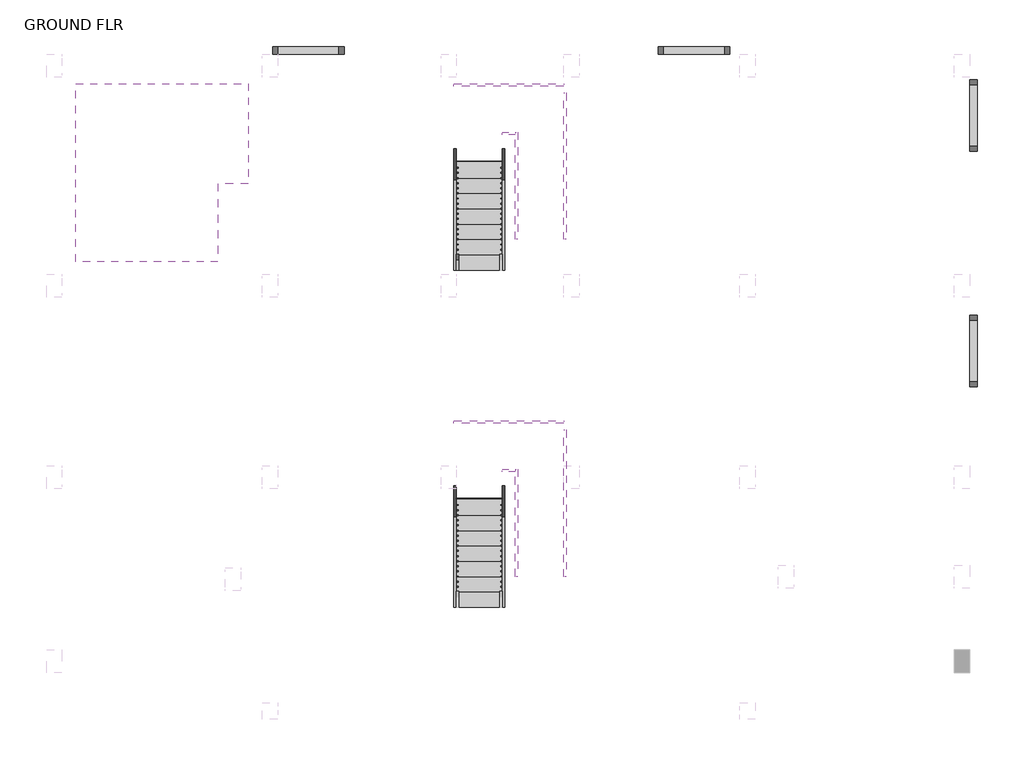
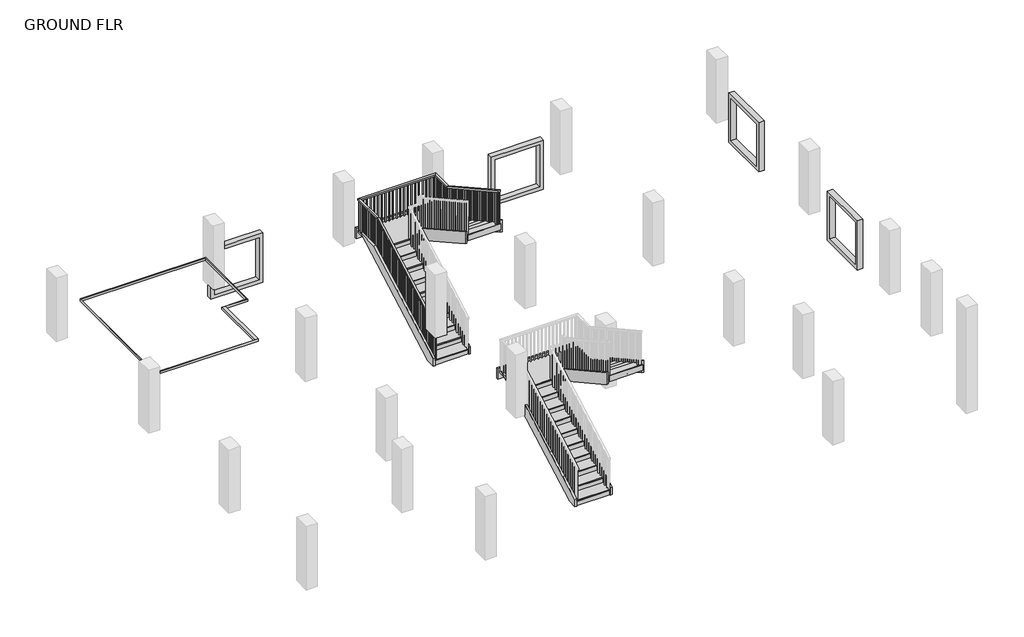
# One storey, part 4 of 4: 12 members, 5 proxies, 2 stair flights, 1 railing.
"""IFC4 building model written with IfcOpenShell, lengths in millimetres."""

from ifc_helpers import new_model, si_unit, frame, origin, place, context, project, spatial, polyline, outline, extrude, faceted_brep, transform, mapped, element, save
from components import generic_models_1_generic_models_1_9ce5a9d9, generic_models_10_generic_models_5_40bb8100, generic_models_13_generic_models_13_6edbfaa0, stair_flight_2b6aeb10, stair_flight_5b78524c

model = new_model("IFC4")

# Units and contexts
model_context = context("Model", 3, world=origin())
ifc_project = project(units=[si_unit("LENGTHUNIT", "METRE", prefix="MILLI")], contexts=[model_context])

# Site, building, storey
site = spatial("IfcSite", under=ifc_project)
building = spatial("IfcBuilding", under=site)
storey = spatial("IfcBuildingStorey", under=building, Name="GROUND FLR", Elevation=304.8)

# Proxies
placement = place(None, origin())
generic_models_1_generic_models_1_shape = generic_models_1_generic_models_1_9ce5a9d9(model_context)
element("IfcBuildingElementProxy", 1, Name="Generic Models 1 : Generic Models 1", ObjectType="Generic Models 1 : Generic Models 1", at=placement, inside=storey, context=model_context, shape_type="MappedRepresentation", body=[
    mapped(generic_models_1_generic_models_1_shape, transform((0.0, 0.0, 0.0), x_axis=(1.0, 0.0, 0.0), y_axis=(0.0, 1.0, 0.0), z_axis=(0.0, 0.0, 1.0))),
])
generic_models_10_generic_models_5_shape = generic_models_10_generic_models_5_40bb8100(model_context)
element("IfcBuildingElementProxy", 2, Name="Generic Models 10 : Generic Models 5", ObjectType="Generic Models 10 : Generic Models 5", at=placement, inside=storey, context=model_context, shape_type="MappedRepresentation", body=[
    mapped(generic_models_10_generic_models_5_shape, transform((0.0, 0.0, -9448.8), x_axis=(1.0, 0.0, 0.0), y_axis=(0.0, 1.0, 0.0), z_axis=(0.0, 0.0, 1.0))),
])
generic_models_13_generic_models_13_shape = generic_models_13_generic_models_13_6edbfaa0(model_context)
element("IfcBuildingElementProxy", 3, Name="Generic Models 19 : Generic Models 13", ObjectType="Generic Models 19 : Generic Models 13", at=placement, inside=storey, context=model_context, shape_type="MappedRepresentation", body=[
    mapped(generic_models_13_generic_models_13_shape, transform((0.0, 0.0, -9448.8), x_axis=(1.0, 0.0, 0.0), y_axis=(0.0, 1.0, 0.0), z_axis=(0.0, 0.0, 1.0))),
])
element("IfcBuildingElementProxy", 4, Name="Generic Models 20 : Generic Models 13", ObjectType="Generic Models 20 : Generic Models 13", at=placement, inside=storey, context=model_context, shape_type="MappedRepresentation", body=[
    mapped(generic_models_13_generic_models_13_shape, transform((-7670.8, 0.0, -9448.8), x_axis=(1.0, 0.0, 0.0), y_axis=(0.0, 1.0, 0.0), z_axis=(0.0, 0.0, 1.0))),
])
element("IfcBuildingElementProxy", 5, Name="Generic Models 9 : Generic Models 5", ObjectType="Generic Models 9 : Generic Models 5", at=placement, inside=storey, context=model_context, shape_type="MappedRepresentation", body=[
    mapped(generic_models_10_generic_models_5_shape, transform((0.0, 4681.8558699, -9448.8), x_axis=(1.0, 0.0, 0.0), y_axis=(0.0, 1.0, 0.0), z_axis=(0.0, 0.0, 1.0))),
])

# Members
element("IfcMember", 6, ObjectType="Stringer - 2\" Width", at=placement, inside=storey, context=model_context, shape_type="SweptSolid", body=[
    extrude(outline(polyline([(-5516.2061634, 304.8), (-5516.2061634, 512.3983948), (-2704.723274, 2074.3333333), (-2077.1016606, 2074.3333333), (-5262.2616606, 304.8), (-5516.2061634, 304.8)])), frame((-1042.9175798, 0.0, 0.0), z_axis=(1.0, 0.0, 0.0), x_axis=(0.0, 1.0, 0.0)), (0.0, 0.0, 1.0), 50.8),
])
element("IfcMember", 7, ObjectType="Stringer - 2\" Width", at=placement, inside=storey, context=model_context, shape_type="SweptSolid", body=[
    extrude(outline(polyline([(-1042.9175798, -1858.6061634), (-1042.9175798, -1807.8061634), (1141.4824202, -1807.8061634), (1141.4824202, -1858.6061634), (-1042.9175798, -1858.6061634)])), frame((0.0, 0.0, 1769.5333333), z_axis=(0.0, 0.0, 1.0), x_axis=(1.0, 0.0, 0.0)), (0.0, 0.0, 1.0), 304.8),
])
element("IfcMember", 8, ObjectType="Stringer - 2\" Width", at=placement, inside=storey, context=model_context, shape_type="SweptSolid", body=[
    extrude(outline(polyline([(-2615.4706662, 1769.5333333), (-4906.6061634, 3042.3863873), (-4906.6061634, 3391.0650614), (-1987.8490528, 1769.5333333), (-2615.4706662, 1769.5333333)])), frame((1141.4824202, 0.0, 0.0), z_axis=(1.0, 0.0, 0.0), x_axis=(0.0, 1.0, 0.0)), (0.0, 0.0, 1.0), 50.8),
])
element("IfcMember", 9, ObjectType="Stringer - 2\" Width", at=placement, inside=storey, context=model_context, shape_type="SweptSolid", body=[
    extrude(outline(polyline([(-5516.2061634, 304.8), (-5516.2061634, 512.3983948), (-2823.8061634, 2008.1761726), (-2823.8061634, 1659.4974984), (-5262.2616606, 304.8), (-5516.2061634, 304.8)])), frame((-77.7175798, 0.0, 0.0), z_axis=(1.0, 0.0, 0.0), x_axis=(0.0, 1.0, 0.0)), (0.0, 0.0, 1.0), 50.8),
])
element("IfcMember", 10, ObjectType="Stringer - 2\" Width", at=placement, inside=storey, context=model_context, shape_type="SweptSolid", body=[
    extrude(outline(polyline([(-77.7175798, -2823.8061634), (-77.7175798, -2773.0061634), (176.2824202, -2773.0061634), (176.2824202, -2823.8061634), (-77.7175798, -2823.8061634)])), frame((0.0, 0.0, 1769.5333333), z_axis=(0.0, 0.0, 1.0), x_axis=(1.0, 0.0, 0.0)), (0.0, 0.0, 1.0), 304.8),
])
element("IfcMember", 11, ObjectType="Stringer - 2\" Width", at=placement, inside=storey, context=model_context, shape_type="SweptSolid", body=[
    extrude(outline(polyline([(-2773.0061634, 2205.7317281), (-2773.0061634, 1857.053054), (-4906.6061634, 3042.3863873), (-4906.6061634, 3391.0650614), (-2773.0061634, 2205.7317281)])), frame((176.2824202, 0.0, 0.0), z_axis=(1.0, 0.0, 0.0), x_axis=(0.0, 1.0, 0.0)), (0.0, 0.0, 1.0), 50.8),
])
element("IfcMember", 12, ObjectType="Stringer - 2\" Width", at=placement, inside=storey, context=model_context, shape_type="SweptSolid", body=[
    extrude(outline(polyline([(-12221.8061634, 304.8), (-12221.8061634, 512.3983948), (-9410.323274, 2074.3333333), (-8782.7016606, 2074.3333333), (-11967.8616606, 304.8), (-12221.8061634, 304.8)])), frame((-1042.9175798, 0.0, 0.0), z_axis=(1.0, 0.0, 0.0), x_axis=(0.0, 1.0, 0.0)), (0.0, 0.0, 1.0), 50.8),
])
element("IfcMember", 13, ObjectType="Stringer - 2\" Width", at=placement, inside=storey, context=model_context, shape_type="SweptSolid", body=[
    extrude(outline(polyline([(-1042.9175798, -8564.2061634), (-1042.9175798, -8513.4061634), (1141.4824202, -8513.4061634), (1141.4824202, -8564.2061634), (-1042.9175798, -8564.2061634)])), frame((0.0, 0.0, 1769.5333333), z_axis=(0.0, 0.0, 1.0), x_axis=(1.0, 0.0, 0.0)), (0.0, 0.0, 1.0), 304.8),
])
element("IfcMember", 14, ObjectType="Stringer - 2\" Width", at=placement, inside=storey, context=model_context, shape_type="SweptSolid", body=[
    extrude(outline(polyline([(-9321.0706662, 1769.5333333), (-11612.2061634, 3042.3863873), (-11612.2061634, 3391.0650614), (-8693.4490528, 1769.5333333), (-9321.0706662, 1769.5333333)])), frame((1141.4824202, 0.0, 0.0), z_axis=(1.0, 0.0, 0.0), x_axis=(0.0, 1.0, 0.0)), (0.0, 0.0, 1.0), 50.8),
])
element("IfcMember", 15, ObjectType="Stringer - 2\" Width", at=placement, inside=storey, context=model_context, shape_type="SweptSolid", body=[
    extrude(outline(polyline([(-12221.8061634, 304.8), (-12221.8061634, 512.3983948), (-9529.4061634, 2008.1761726), (-9529.4061634, 1659.4974984), (-11967.8616606, 304.8), (-12221.8061634, 304.8)])), frame((-77.7175798, 0.0, 0.0), z_axis=(1.0, 0.0, 0.0), x_axis=(0.0, 1.0, 0.0)), (0.0, 0.0, 1.0), 50.8),
])
element("IfcMember", 16, ObjectType="Stringer - 2\" Width", at=placement, inside=storey, context=model_context, shape_type="SweptSolid", body=[
    extrude(outline(polyline([(-77.7175798, -9529.4061634), (-77.7175798, -9478.6061634), (176.2824202, -9478.6061634), (176.2824202, -9529.4061634), (-77.7175798, -9529.4061634)])), frame((0.0, 0.0, 1769.5333333), z_axis=(0.0, 0.0, 1.0), x_axis=(1.0, 0.0, 0.0)), (0.0, 0.0, 1.0), 304.8),
])
element("IfcMember", 17, ObjectType="Stringer - 2\" Width", at=placement, inside=storey, context=model_context, shape_type="SweptSolid", body=[
    extrude(outline(polyline([(-9478.6061634, 2205.7317281), (-9478.6061634, 1857.053054), (-11612.2061634, 3042.3863873), (-11612.2061634, 3391.0650614), (-9478.6061634, 2205.7317281)])), frame((176.2824202, 0.0, 0.0), z_axis=(1.0, 0.0, 0.0), x_axis=(0.0, 1.0, 0.0)), (0.0, 0.0, 1.0), 50.8),
])

# Railing
element("IfcRailing", 18, ObjectType="Handrail - Rectangular", at=placement, inside=storey, context=model_context, shape_type="SolidModel", body=[
    faceted_brep([(-992.1175798, -5516.2061634, 1388.5333333), (-992.1175798, -5516.2061634, 1330.420221), (-941.3175798, -5516.2061634, 1330.420221), (-941.3175798, -5516.2061634, 1388.5333333), (-992.1175798, -2773.0061634, 2912.5333333), (-992.1175798, -2759.8425611, 2861.7333333), (-941.3175798, -2759.8425611, 2861.7333333), (-941.3175798, -2773.0061634, 2912.5333333), (-992.1175798, -1858.6061634, 2912.5333333), (-992.1175798, -1858.6061634, 2861.7333333), (-941.3175798, -1909.4061634, 2861.7333333), (-941.3175798, -1909.4061634, 2912.5333333), (1141.4824202, -1858.6061634, 2912.5333333), (1141.4824202, -1858.6061634, 2861.7333333), (1090.6824202, -1909.4061634, 2861.7333333), (1090.6824202, -1909.4061634, 2912.5333333), (1141.4824202, -2468.2061634, 2912.5333333), (1141.4824202, -2481.3697656, 2861.7333333), (1090.6824202, -2481.3697656, 2861.7333333), (1090.6824202, -2468.2061634, 2912.5333333), (1141.4824202, -4906.6061634, 4267.2), (1090.6824202, -4906.6061634, 4267.2), (1090.6824202, -4906.6061634, 4209.0868876), (1141.4824202, -4906.6061634, 4209.0868876)], [[[0, 1, 2, 3]], [[1, 0, 4, 5]], [[2, 1, 5, 6]], [[3, 2, 6, 7]], [[0, 3, 7, 4]], [[5, 4, 8, 9]], [[6, 5, 9, 10]], [[7, 6, 10, 11]], [[4, 7, 11, 8]], [[9, 8, 12, 13]], [[10, 9, 13, 14]], [[11, 10, 14, 15]], [[8, 11, 15, 12]], [[13, 12, 16, 17]], [[14, 13, 17, 18]], [[15, 14, 18, 19]], [[12, 15, 19, 16]], [[20, 21, 22, 23]], [[17, 16, 20, 23]], [[18, 17, 23, 22]], [[19, 18, 22, 21]], [[16, 19, 21, 20]]]),
    extrude(outline(polyline([(-4820.8811634, 4161.4618876), (-4820.8811634, 3183.4666667), (-4839.9311634, 3183.4666667), (-4839.9311634, 4172.045221), (-4820.8811634, 4161.4618876)])), frame((1106.5574202, 0.0, 0.0), z_axis=(1.0, 0.0, 0.0), x_axis=(0.0, 1.0, 0.0)), (0.0, 0.0, 1.0), 19.05),
    extrude(outline(polyline([(-4719.2811634, 4105.0174432), (-4719.2811634, 3183.4666667), (-4738.3311634, 3183.4666667), (-4738.3311634, 4115.6007765), (-4719.2811634, 4105.0174432)])), frame((1106.5574202, 0.0, 0.0), z_axis=(1.0, 0.0, 0.0), x_axis=(0.0, 1.0, 0.0)), (0.0, 0.0, 1.0), 19.05),
    extrude(outline(polyline([(-4617.6811634, 4048.5729988), (-4617.6811634, 3183.4666667), (-4636.7311634, 3183.4666667), (-4636.7311634, 4059.1563321), (-4617.6811634, 4048.5729988)])), frame((1106.5574202, 0.0, 0.0), z_axis=(1.0, 0.0, 0.0), x_axis=(0.0, 1.0, 0.0)), (0.0, 0.0, 1.0), 19.05),
    extrude(outline(polyline([(-4516.0811634, 3992.1285543), (-4516.0811634, 3014.1333333), (-4535.1311634, 3014.1333333), (-4535.1311634, 4002.7118876), (-4516.0811634, 3992.1285543)])), frame((1106.5574202, 0.0, 0.0), z_axis=(1.0, 0.0, 0.0), x_axis=(0.0, 1.0, 0.0)), (0.0, 0.0, 1.0), 19.05),
    extrude(outline(polyline([(-4414.4811634, 3935.6841099), (-4414.4811634, 3014.1333333), (-4433.5311634, 3014.1333333), (-4433.5311634, 3946.2674432), (-4414.4811634, 3935.6841099)])), frame((1106.5574202, 0.0, 0.0), z_axis=(1.0, 0.0, 0.0), x_axis=(0.0, 1.0, 0.0)), (0.0, 0.0, 1.0), 19.05),
    extrude(outline(polyline([(-4312.8811634, 3879.2396654), (-4312.8811634, 3014.1333333), (-4331.9311634, 3014.1333333), (-4331.9311634, 3889.8229988), (-4312.8811634, 3879.2396654)])), frame((1106.5574202, 0.0, 0.0), z_axis=(1.0, 0.0, 0.0), x_axis=(0.0, 1.0, 0.0)), (0.0, 0.0, 1.0), 19.05),
    extrude(outline(polyline([(-4211.2811634, 3822.795221), (-4211.2811634, 2844.8), (-4230.3311634, 2844.8), (-4230.3311634, 3833.3785543), (-4211.2811634, 3822.795221)])), frame((1106.5574202, 0.0, 0.0), z_axis=(1.0, 0.0, 0.0), x_axis=(0.0, 1.0, 0.0)), (0.0, 0.0, 1.0), 19.05),
    extrude(outline(polyline([(-4109.6811634, 3766.3507765), (-4109.6811634, 2844.8), (-4128.7311634, 2844.8), (-4128.7311634, 3776.9341099), (-4109.6811634, 3766.3507765)])), frame((1106.5574202, 0.0, 0.0), z_axis=(1.0, 0.0, 0.0), x_axis=(0.0, 1.0, 0.0)), (0.0, 0.0, 1.0), 19.05),
    extrude(outline(polyline([(-4008.0811634, 3709.9063321), (-4008.0811634, 2844.8), (-4027.1311634, 2844.8), (-4027.1311634, 3720.4896654), (-4008.0811634, 3709.9063321)])), frame((1106.5574202, 0.0, 0.0), z_axis=(1.0, 0.0, 0.0), x_axis=(0.0, 1.0, 0.0)), (0.0, 0.0, 1.0), 19.05),
    extrude(outline(polyline([(-3906.4811634, 3653.4618876), (-3906.4811634, 2675.4666667), (-3925.5311634, 2675.4666667), (-3925.5311634, 3664.045221), (-3906.4811634, 3653.4618876)])), frame((1106.5574202, 0.0, 0.0), z_axis=(1.0, 0.0, 0.0), x_axis=(0.0, 1.0, 0.0)), (0.0, 0.0, 1.0), 19.05),
    extrude(outline(polyline([(-3804.8811634, 3597.0174432), (-3804.8811634, 2675.4666667), (-3823.9311634, 2675.4666667), (-3823.9311634, 3607.6007765), (-3804.8811634, 3597.0174432)])), frame((1106.5574202, 0.0, 0.0), z_axis=(1.0, 0.0, 0.0), x_axis=(0.0, 1.0, 0.0)), (0.0, 0.0, 1.0), 19.05),
    extrude(outline(polyline([(-3703.2811634, 3540.5729988), (-3703.2811634, 2675.4666667), (-3722.3311634, 2675.4666667), (-3722.3311634, 3551.1563321), (-3703.2811634, 3540.5729988)])), frame((1106.5574202, 0.0, 0.0), z_axis=(1.0, 0.0, 0.0), x_axis=(0.0, 1.0, 0.0)), (0.0, 0.0, 1.0), 19.05),
    extrude(outline(polyline([(-3601.6811634, 3484.1285543), (-3601.6811634, 2506.1333333), (-3620.7311634, 2506.1333333), (-3620.7311634, 3494.7118876), (-3601.6811634, 3484.1285543)])), frame((1106.5574202, 0.0, 0.0), z_axis=(1.0, 0.0, 0.0), x_axis=(0.0, 1.0, 0.0)), (0.0, 0.0, 1.0), 19.05),
    extrude(outline(polyline([(-3500.0811634, 3427.6841099), (-3500.0811634, 2506.1333333), (-3519.1311634, 2506.1333333), (-3519.1311634, 3438.2674432), (-3500.0811634, 3427.6841099)])), frame((1106.5574202, 0.0, 0.0), z_axis=(1.0, 0.0, 0.0), x_axis=(0.0, 1.0, 0.0)), (0.0, 0.0, 1.0), 19.05),
    extrude(outline(polyline([(-3398.4811634, 3371.2396654), (-3398.4811634, 2506.1333333), (-3417.5311634, 2506.1333333), (-3417.5311634, 3381.8229988), (-3398.4811634, 3371.2396654)])), frame((1106.5574202, 0.0, 0.0), z_axis=(1.0, 0.0, 0.0), x_axis=(0.0, 1.0, 0.0)), (0.0, 0.0, 1.0), 19.05),
    extrude(outline(polyline([(-3296.8811634, 3314.795221), (-3296.8811634, 2336.8), (-3315.9311634, 2336.8), (-3315.9311634, 3325.3785543), (-3296.8811634, 3314.795221)])), frame((1106.5574202, 0.0, 0.0), z_axis=(1.0, 0.0, 0.0), x_axis=(0.0, 1.0, 0.0)), (0.0, 0.0, 1.0), 19.05),
    extrude(outline(polyline([(-3195.2811634, 3258.3507765), (-3195.2811634, 2336.8), (-3214.3311634, 2336.8), (-3214.3311634, 3268.9341099), (-3195.2811634, 3258.3507765)])), frame((1106.5574202, 0.0, 0.0), z_axis=(1.0, 0.0, 0.0), x_axis=(0.0, 1.0, 0.0)), (0.0, 0.0, 1.0), 19.05),
    extrude(outline(polyline([(-3093.6811634, 3201.9063321), (-3093.6811634, 2336.8), (-3112.7311634, 2336.8), (-3112.7311634, 3212.4896654), (-3093.6811634, 3201.9063321)])), frame((1106.5574202, 0.0, 0.0), z_axis=(1.0, 0.0, 0.0), x_axis=(0.0, 1.0, 0.0)), (0.0, 0.0, 1.0), 19.05),
    extrude(outline(polyline([(-2992.0811634, 3145.4618876), (-2992.0811634, 2167.4666667), (-3011.1311634, 2167.4666667), (-3011.1311634, 3156.045221), (-2992.0811634, 3145.4618876)])), frame((1106.5574202, 0.0, 0.0), z_axis=(1.0, 0.0, 0.0), x_axis=(0.0, 1.0, 0.0)), (0.0, 0.0, 1.0), 19.05),
    extrude(outline(polyline([(-2890.4811634, 3089.0174432), (-2890.4811634, 2167.4666667), (-2909.5311634, 2167.4666667), (-2909.5311634, 3099.6007765), (-2890.4811634, 3089.0174432)])), frame((1106.5574202, 0.0, 0.0), z_axis=(1.0, 0.0, 0.0), x_axis=(0.0, 1.0, 0.0)), (0.0, 0.0, 1.0), 19.05),
    extrude(outline(polyline([(-2788.8811634, 3032.5729988), (-2788.8811634, 2167.4666667), (-2807.9311634, 2167.4666667), (-2807.9311634, 3043.1563321), (-2788.8811634, 3032.5729988)])), frame((1106.5574202, 0.0, 0.0), z_axis=(1.0, 0.0, 0.0), x_axis=(0.0, 1.0, 0.0)), (0.0, 0.0, 1.0), 19.05),
    extrude(outline(polyline([(-2687.2811634, 2976.1285543), (-2687.2811634, 1998.1333333), (-2706.3311634, 1998.1333333), (-2706.3311634, 2986.7118876), (-2687.2811634, 2976.1285543)])), frame((1106.5574202, 0.0, 0.0), z_axis=(1.0, 0.0, 0.0), x_axis=(0.0, 1.0, 0.0)), (0.0, 0.0, 1.0), 19.05),
    extrude(outline(polyline([(-2585.6811634, 2919.6841099), (-2585.6811634, 1998.1333333), (-2604.7311634, 1998.1333333), (-2604.7311634, 2930.2674432), (-2585.6811634, 2919.6841099)])), frame((1106.5574202, 0.0, 0.0), z_axis=(1.0, 0.0, 0.0), x_axis=(0.0, 1.0, 0.0)), (0.0, 0.0, 1.0), 19.05),
    extrude(outline(polyline([(-2484.0811634, 2863.2396654), (-2484.0811634, 1998.1333333), (-2503.1311634, 1998.1333333), (-2503.1311634, 2873.8229988), (-2484.0811634, 2863.2396654)])), frame((1106.5574202, 0.0, 0.0), z_axis=(1.0, 0.0, 0.0), x_axis=(0.0, 1.0, 0.0)), (0.0, 0.0, 1.0), 19.05),
    extrude(outline(polyline([(1125.6074202, -2382.4811634), (1125.6074202, -2401.5311634), (1106.5574202, -2401.5311634), (1106.5574202, -2382.4811634), (1125.6074202, -2382.4811634)])), frame((0.0, 0.0, 1998.1333333), z_axis=(0.0, 0.0, 1.0), x_axis=(1.0, 0.0, 0.0)), (0.0, 0.0, 1.0), 863.6),
    extrude(outline(polyline([(1125.6074202, -2280.8811634), (1125.6074202, -2299.9311634), (1106.5574202, -2299.9311634), (1106.5574202, -2280.8811634), (1125.6074202, -2280.8811634)])), frame((0.0, 0.0, 1998.1333333), z_axis=(0.0, 0.0, 1.0), x_axis=(1.0, 0.0, 0.0)), (0.0, 0.0, 1.0), 863.6),
    extrude(outline(polyline([(1125.6074202, -2179.2811634), (1125.6074202, -2198.3311634), (1106.5574202, -2198.3311634), (1106.5574202, -2179.2811634), (1125.6074202, -2179.2811634)])), frame((0.0, 0.0, 1998.1333333), z_axis=(0.0, 0.0, 1.0), x_axis=(1.0, 0.0, 0.0)), (0.0, 0.0, 1.0), 863.6),
    extrude(outline(polyline([(1125.6074202, -2077.6811634), (1125.6074202, -2096.7311634), (1106.5574202, -2096.7311634), (1106.5574202, -2077.6811634), (1125.6074202, -2077.6811634)])), frame((0.0, 0.0, 1998.1333333), z_axis=(0.0, 0.0, 1.0), x_axis=(1.0, 0.0, 0.0)), (0.0, 0.0, 1.0), 863.6),
    extrude(outline(polyline([(1125.6074202, -1976.0811634), (1125.6074202, -1995.1311634), (1106.5574202, -1995.1311634), (1106.5574202, -1976.0811634), (1125.6074202, -1976.0811634)])), frame((0.0, 0.0, 1998.1333333), z_axis=(0.0, 0.0, 1.0), x_axis=(1.0, 0.0, 0.0)), (0.0, 0.0, 1.0), 863.6),
    extrude(outline(polyline([(1055.7574202, -1874.4811634), (1074.8074202, -1874.4811634), (1074.8074202, -1893.5311634), (1055.7574202, -1893.5311634), (1055.7574202, -1874.4811634)])), frame((0.0, 0.0, 1998.1333333), z_axis=(0.0, 0.0, 1.0), x_axis=(1.0, 0.0, 0.0)), (0.0, 0.0, 1.0), 863.6),
    extrude(outline(polyline([(954.1574202, -1874.4811634), (973.2074202, -1874.4811634), (973.2074202, -1893.5311634), (954.1574202, -1893.5311634), (954.1574202, -1874.4811634)])), frame((0.0, 0.0, 1998.1333333), z_axis=(0.0, 0.0, 1.0), x_axis=(1.0, 0.0, 0.0)), (0.0, 0.0, 1.0), 863.6),
    extrude(outline(polyline([(852.5574202, -1874.4811634), (871.6074202, -1874.4811634), (871.6074202, -1893.5311634), (852.5574202, -1893.5311634), (852.5574202, -1874.4811634)])), frame((0.0, 0.0, 1998.1333333), z_axis=(0.0, 0.0, 1.0), x_axis=(1.0, 0.0, 0.0)), (0.0, 0.0, 1.0), 863.6),
    extrude(outline(polyline([(750.9574202, -1874.4811634), (770.0074202, -1874.4811634), (770.0074202, -1893.5311634), (750.9574202, -1893.5311634), (750.9574202, -1874.4811634)])), frame((0.0, 0.0, 1998.1333333), z_axis=(0.0, 0.0, 1.0), x_axis=(1.0, 0.0, 0.0)), (0.0, 0.0, 1.0), 863.6),
    extrude(outline(polyline([(649.3574202, -1874.4811634), (668.4074202, -1874.4811634), (668.4074202, -1893.5311634), (649.3574202, -1893.5311634), (649.3574202, -1874.4811634)])), frame((0.0, 0.0, 1998.1333333), z_axis=(0.0, 0.0, 1.0), x_axis=(1.0, 0.0, 0.0)), (0.0, 0.0, 1.0), 863.6),
    extrude(outline(polyline([(547.7574202, -1874.4811634), (566.8074202, -1874.4811634), (566.8074202, -1893.5311634), (547.7574202, -1893.5311634), (547.7574202, -1874.4811634)])), frame((0.0, 0.0, 1998.1333333), z_axis=(0.0, 0.0, 1.0), x_axis=(1.0, 0.0, 0.0)), (0.0, 0.0, 1.0), 863.6),
    extrude(outline(polyline([(446.1574202, -1874.4811634), (465.2074202, -1874.4811634), (465.2074202, -1893.5311634), (446.1574202, -1893.5311634), (446.1574202, -1874.4811634)])), frame((0.0, 0.0, 1998.1333333), z_axis=(0.0, 0.0, 1.0), x_axis=(1.0, 0.0, 0.0)), (0.0, 0.0, 1.0), 863.6),
    extrude(outline(polyline([(344.5574202, -1874.4811634), (363.6074202, -1874.4811634), (363.6074202, -1893.5311634), (344.5574202, -1893.5311634), (344.5574202, -1874.4811634)])), frame((0.0, 0.0, 1998.1333333), z_axis=(0.0, 0.0, 1.0), x_axis=(1.0, 0.0, 0.0)), (0.0, 0.0, 1.0), 863.6),
    extrude(outline(polyline([(242.9574202, -1874.4811634), (262.0074202, -1874.4811634), (262.0074202, -1893.5311634), (242.9574202, -1893.5311634), (242.9574202, -1874.4811634)])), frame((0.0, 0.0, 1998.1333333), z_axis=(0.0, 0.0, 1.0), x_axis=(1.0, 0.0, 0.0)), (0.0, 0.0, 1.0), 863.6),
    extrude(outline(polyline([(141.3574202, -1874.4811634), (160.4074202, -1874.4811634), (160.4074202, -1893.5311634), (141.3574202, -1893.5311634), (141.3574202, -1874.4811634)])), frame((0.0, 0.0, 1998.1333333), z_axis=(0.0, 0.0, 1.0), x_axis=(1.0, 0.0, 0.0)), (0.0, 0.0, 1.0), 863.6),
    extrude(outline(polyline([(39.7574202, -1874.4811634), (58.8074202, -1874.4811634), (58.8074202, -1893.5311634), (39.7574202, -1893.5311634), (39.7574202, -1874.4811634)])), frame((0.0, 0.0, 1998.1333333), z_axis=(0.0, 0.0, 1.0), x_axis=(1.0, 0.0, 0.0)), (0.0, 0.0, 1.0), 863.6),
    extrude(outline(polyline([(-61.8425798, -1874.4811634), (-42.7925798, -1874.4811634), (-42.7925798, -1893.5311634), (-61.8425798, -1893.5311634), (-61.8425798, -1874.4811634)])), frame((0.0, 0.0, 1998.1333333), z_axis=(0.0, 0.0, 1.0), x_axis=(1.0, 0.0, 0.0)), (0.0, 0.0, 1.0), 863.6),
    extrude(outline(polyline([(-163.4425798, -1874.4811634), (-144.3925798, -1874.4811634), (-144.3925798, -1893.5311634), (-163.4425798, -1893.5311634), (-163.4425798, -1874.4811634)])), frame((0.0, 0.0, 1998.1333333), z_axis=(0.0, 0.0, 1.0), x_axis=(1.0, 0.0, 0.0)), (0.0, 0.0, 1.0), 863.6),
    extrude(outline(polyline([(-265.0425798, -1874.4811634), (-245.9925798, -1874.4811634), (-245.9925798, -1893.5311634), (-265.0425798, -1893.5311634), (-265.0425798, -1874.4811634)])), frame((0.0, 0.0, 1998.1333333), z_axis=(0.0, 0.0, 1.0), x_axis=(1.0, 0.0, 0.0)), (0.0, 0.0, 1.0), 863.6),
    extrude(outline(polyline([(-366.6425798, -1874.4811634), (-347.5925798, -1874.4811634), (-347.5925798, -1893.5311634), (-366.6425798, -1893.5311634), (-366.6425798, -1874.4811634)])), frame((0.0, 0.0, 1998.1333333), z_axis=(0.0, 0.0, 1.0), x_axis=(1.0, 0.0, 0.0)), (0.0, 0.0, 1.0), 863.6),
    extrude(outline(polyline([(-468.2425798, -1874.4811634), (-449.1925798, -1874.4811634), (-449.1925798, -1893.5311634), (-468.2425798, -1893.5311634), (-468.2425798, -1874.4811634)])), frame((0.0, 0.0, 1998.1333333), z_axis=(0.0, 0.0, 1.0), x_axis=(1.0, 0.0, 0.0)), (0.0, 0.0, 1.0), 863.6),
    extrude(outline(polyline([(-569.8425798, -1874.4811634), (-550.7925798, -1874.4811634), (-550.7925798, -1893.5311634), (-569.8425798, -1893.5311634), (-569.8425798, -1874.4811634)])), frame((0.0, 0.0, 1998.1333333), z_axis=(0.0, 0.0, 1.0), x_axis=(1.0, 0.0, 0.0)), (0.0, 0.0, 1.0), 863.6),
    extrude(outline(polyline([(-671.4425798, -1874.4811634), (-652.3925798, -1874.4811634), (-652.3925798, -1893.5311634), (-671.4425798, -1893.5311634), (-671.4425798, -1874.4811634)])), frame((0.0, 0.0, 1998.1333333), z_axis=(0.0, 0.0, 1.0), x_axis=(1.0, 0.0, 0.0)), (0.0, 0.0, 1.0), 863.6),
    extrude(outline(polyline([(-773.0425798, -1874.4811634), (-753.9925798, -1874.4811634), (-753.9925798, -1893.5311634), (-773.0425798, -1893.5311634), (-773.0425798, -1874.4811634)])), frame((0.0, 0.0, 1998.1333333), z_axis=(0.0, 0.0, 1.0), x_axis=(1.0, 0.0, 0.0)), (0.0, 0.0, 1.0), 863.6),
    extrude(outline(polyline([(-874.6425798, -1874.4811634), (-855.5925798, -1874.4811634), (-855.5925798, -1893.5311634), (-874.6425798, -1893.5311634), (-874.6425798, -1874.4811634)])), frame((0.0, 0.0, 1998.1333333), z_axis=(0.0, 0.0, 1.0), x_axis=(1.0, 0.0, 0.0)), (0.0, 0.0, 1.0), 863.6),
    extrude(outline(polyline([(-976.2425798, -1969.7311634), (-976.2425798, -1950.6811634), (-957.1925798, -1950.6811634), (-957.1925798, -1969.7311634), (-976.2425798, -1969.7311634)])), frame((0.0, 0.0, 1998.1333333), z_axis=(0.0, 0.0, 1.0), x_axis=(1.0, 0.0, 0.0)), (0.0, 0.0, 1.0), 863.6),
    extrude(outline(polyline([(-976.2425798, -2071.3311634), (-976.2425798, -2052.2811634), (-957.1925798, -2052.2811634), (-957.1925798, -2071.3311634), (-976.2425798, -2071.3311634)])), frame((0.0, 0.0, 1998.1333333), z_axis=(0.0, 0.0, 1.0), x_axis=(1.0, 0.0, 0.0)), (0.0, 0.0, 1.0), 863.6),
    extrude(outline(polyline([(-976.2425798, -2172.9311634), (-976.2425798, -2153.8811634), (-957.1925798, -2153.8811634), (-957.1925798, -2172.9311634), (-976.2425798, -2172.9311634)])), frame((0.0, 0.0, 1998.1333333), z_axis=(0.0, 0.0, 1.0), x_axis=(1.0, 0.0, 0.0)), (0.0, 0.0, 1.0), 863.6),
    extrude(outline(polyline([(-976.2425798, -2274.5311634), (-976.2425798, -2255.4811634), (-957.1925798, -2255.4811634), (-957.1925798, -2274.5311634), (-976.2425798, -2274.5311634)])), frame((0.0, 0.0, 1998.1333333), z_axis=(0.0, 0.0, 1.0), x_axis=(1.0, 0.0, 0.0)), (0.0, 0.0, 1.0), 863.6),
    extrude(outline(polyline([(-976.2425798, -2376.1311634), (-976.2425798, -2357.0811634), (-957.1925798, -2357.0811634), (-957.1925798, -2376.1311634), (-976.2425798, -2376.1311634)])), frame((0.0, 0.0, 1998.1333333), z_axis=(0.0, 0.0, 1.0), x_axis=(1.0, 0.0, 0.0)), (0.0, 0.0, 1.0), 863.6),
    extrude(outline(polyline([(-976.2425798, -2477.7311634), (-976.2425798, -2458.6811634), (-957.1925798, -2458.6811634), (-957.1925798, -2477.7311634), (-976.2425798, -2477.7311634)])), frame((0.0, 0.0, 1998.1333333), z_axis=(0.0, 0.0, 1.0), x_axis=(1.0, 0.0, 0.0)), (0.0, 0.0, 1.0), 863.6),
    extrude(outline(polyline([(-976.2425798, -2579.3311634), (-976.2425798, -2560.2811634), (-957.1925798, -2560.2811634), (-957.1925798, -2579.3311634), (-976.2425798, -2579.3311634)])), frame((0.0, 0.0, 1998.1333333), z_axis=(0.0, 0.0, 1.0), x_axis=(1.0, 0.0, 0.0)), (0.0, 0.0, 1.0), 863.6),
    extrude(outline(polyline([(-976.2425798, -2680.9311634), (-976.2425798, -2661.8811634), (-957.1925798, -2661.8811634), (-957.1925798, -2680.9311634), (-976.2425798, -2680.9311634)])), frame((0.0, 0.0, 1998.1333333), z_axis=(0.0, 0.0, 1.0), x_axis=(1.0, 0.0, 0.0)), (0.0, 0.0, 1.0), 863.6),
    extrude(outline(polyline([(-2763.4811634, 2859.7118876), (-2763.4811634, 1998.1333333), (-2782.5311634, 1998.1333333), (-2782.5311634, 2849.1285543), (-2763.4811634, 2859.7118876)])), frame((-976.2425798, 0.0, 0.0), z_axis=(1.0, 0.0, 0.0), x_axis=(0.0, 1.0, 0.0)), (0.0, 0.0, 1.0), 19.05),
    extrude(outline(polyline([(-2865.0811634, 2803.2674432), (-2865.0811634, 1828.8), (-2884.1311634, 1828.8), (-2884.1311634, 2792.6841099), (-2865.0811634, 2803.2674432)])), frame((-976.2425798, 0.0, 0.0), z_axis=(1.0, 0.0, 0.0), x_axis=(0.0, 1.0, 0.0)), (0.0, 0.0, 1.0), 19.05),
    extrude(outline(polyline([(-2966.6811634, 2746.8229988), (-2966.6811634, 1828.8), (-2985.7311634, 1828.8), (-2985.7311634, 2736.2396654), (-2966.6811634, 2746.8229988)])), frame((-976.2425798, 0.0, 0.0), z_axis=(1.0, 0.0, 0.0), x_axis=(0.0, 1.0, 0.0)), (0.0, 0.0, 1.0), 19.05),
    extrude(outline(polyline([(-3068.2811634, 2690.3785543), (-3068.2811634, 1828.8), (-3087.3311634, 1828.8), (-3087.3311634, 2679.795221), (-3068.2811634, 2690.3785543)])), frame((-976.2425798, 0.0, 0.0), z_axis=(1.0, 0.0, 0.0), x_axis=(0.0, 1.0, 0.0)), (0.0, 0.0, 1.0), 19.05),
    extrude(outline(polyline([(-3169.8811634, 2633.9341099), (-3169.8811634, 1659.4666667), (-3188.9311634, 1659.4666667), (-3188.9311634, 2623.3507765), (-3169.8811634, 2633.9341099)])), frame((-976.2425798, 0.0, 0.0), z_axis=(1.0, 0.0, 0.0), x_axis=(0.0, 1.0, 0.0)), (0.0, 0.0, 1.0), 19.05),
    extrude(outline(polyline([(-3271.4811634, 2577.4896654), (-3271.4811634, 1659.4666667), (-3290.5311634, 1659.4666667), (-3290.5311634, 2566.9063321), (-3271.4811634, 2577.4896654)])), frame((-976.2425798, 0.0, 0.0), z_axis=(1.0, 0.0, 0.0), x_axis=(0.0, 1.0, 0.0)), (0.0, 0.0, 1.0), 19.05),
    extrude(outline(polyline([(-3373.0811634, 2521.045221), (-3373.0811634, 1659.4666667), (-3392.1311634, 1659.4666667), (-3392.1311634, 2510.4618876), (-3373.0811634, 2521.045221)])), frame((-976.2425798, 0.0, 0.0), z_axis=(1.0, 0.0, 0.0), x_axis=(0.0, 1.0, 0.0)), (0.0, 0.0, 1.0), 19.05),
    extrude(outline(polyline([(-3474.6811634, 2464.6007765), (-3474.6811634, 1490.1333333), (-3493.7311634, 1490.1333333), (-3493.7311634, 2454.0174432), (-3474.6811634, 2464.6007765)])), frame((-976.2425798, 0.0, 0.0), z_axis=(1.0, 0.0, 0.0), x_axis=(0.0, 1.0, 0.0)), (0.0, 0.0, 1.0), 19.05),
    extrude(outline(polyline([(-3576.2811634, 2408.1563321), (-3576.2811634, 1490.1333333), (-3595.3311634, 1490.1333333), (-3595.3311634, 2397.5729988), (-3576.2811634, 2408.1563321)])), frame((-976.2425798, 0.0, 0.0), z_axis=(1.0, 0.0, 0.0), x_axis=(0.0, 1.0, 0.0)), (0.0, 0.0, 1.0), 19.05),
    extrude(outline(polyline([(-3677.8811634, 2351.7118876), (-3677.8811634, 1490.1333333), (-3696.9311634, 1490.1333333), (-3696.9311634, 2341.1285543), (-3677.8811634, 2351.7118876)])), frame((-976.2425798, 0.0, 0.0), z_axis=(1.0, 0.0, 0.0), x_axis=(0.0, 1.0, 0.0)), (0.0, 0.0, 1.0), 19.05),
    extrude(outline(polyline([(-3779.4811634, 2295.2674432), (-3779.4811634, 1320.8), (-3798.5311634, 1320.8), (-3798.5311634, 2284.6841099), (-3779.4811634, 2295.2674432)])), frame((-976.2425798, 0.0, 0.0), z_axis=(1.0, 0.0, 0.0), x_axis=(0.0, 1.0, 0.0)), (0.0, 0.0, 1.0), 19.05),
    extrude(outline(polyline([(-3881.0811634, 2238.8229988), (-3881.0811634, 1320.8), (-3900.1311634, 1320.8), (-3900.1311634, 2228.2396654), (-3881.0811634, 2238.8229988)])), frame((-976.2425798, 0.0, 0.0), z_axis=(1.0, 0.0, 0.0), x_axis=(0.0, 1.0, 0.0)), (0.0, 0.0, 1.0), 19.05),
    extrude(outline(polyline([(-3982.6811634, 2182.3785543), (-3982.6811634, 1320.8), (-4001.7311634, 1320.8), (-4001.7311634, 2171.795221), (-3982.6811634, 2182.3785543)])), frame((-976.2425798, 0.0, 0.0), z_axis=(1.0, 0.0, 0.0), x_axis=(0.0, 1.0, 0.0)), (0.0, 0.0, 1.0), 19.05),
    extrude(outline(polyline([(-4084.2811634, 2125.9341099), (-4084.2811634, 1151.4666667), (-4103.3311634, 1151.4666667), (-4103.3311634, 2115.3507765), (-4084.2811634, 2125.9341099)])), frame((-976.2425798, 0.0, 0.0), z_axis=(1.0, 0.0, 0.0), x_axis=(0.0, 1.0, 0.0)), (0.0, 0.0, 1.0), 19.05),
    extrude(outline(polyline([(-4185.8811634, 2069.4896654), (-4185.8811634, 1151.4666667), (-4204.9311634, 1151.4666667), (-4204.9311634, 2058.9063321), (-4185.8811634, 2069.4896654)])), frame((-976.2425798, 0.0, 0.0), z_axis=(1.0, 0.0, 0.0), x_axis=(0.0, 1.0, 0.0)), (0.0, 0.0, 1.0), 19.05),
    extrude(outline(polyline([(-4287.4811634, 2013.045221), (-4287.4811634, 1151.4666667), (-4306.5311634, 1151.4666667), (-4306.5311634, 2002.4618876), (-4287.4811634, 2013.045221)])), frame((-976.2425798, 0.0, 0.0), z_axis=(1.0, 0.0, 0.0), x_axis=(0.0, 1.0, 0.0)), (0.0, 0.0, 1.0), 19.05),
    extrude(outline(polyline([(-4389.0811634, 1956.6007765), (-4389.0811634, 982.1333333), (-4408.1311634, 982.1333333), (-4408.1311634, 1946.0174432), (-4389.0811634, 1956.6007765)])), frame((-976.2425798, 0.0, 0.0), z_axis=(1.0, 0.0, 0.0), x_axis=(0.0, 1.0, 0.0)), (0.0, 0.0, 1.0), 19.05),
    extrude(outline(polyline([(-4490.6811634, 1900.1563321), (-4490.6811634, 982.1333333), (-4509.7311634, 982.1333333), (-4509.7311634, 1889.5729988), (-4490.6811634, 1900.1563321)])), frame((-976.2425798, 0.0, 0.0), z_axis=(1.0, 0.0, 0.0), x_axis=(0.0, 1.0, 0.0)), (0.0, 0.0, 1.0), 19.05),
    extrude(outline(polyline([(-4592.2811634, 1843.7118876), (-4592.2811634, 982.1333333), (-4611.3311634, 982.1333333), (-4611.3311634, 1833.1285543), (-4592.2811634, 1843.7118876)])), frame((-976.2425798, 0.0, 0.0), z_axis=(1.0, 0.0, 0.0), x_axis=(0.0, 1.0, 0.0)), (0.0, 0.0, 1.0), 19.05),
    extrude(outline(polyline([(-4693.8811634, 1787.2674432), (-4693.8811634, 812.8), (-4712.9311634, 812.8), (-4712.9311634, 1776.6841099), (-4693.8811634, 1787.2674432)])), frame((-976.2425798, 0.0, 0.0), z_axis=(1.0, 0.0, 0.0), x_axis=(0.0, 1.0, 0.0)), (0.0, 0.0, 1.0), 19.05),
    extrude(outline(polyline([(-4795.4811634, 1730.8229988), (-4795.4811634, 812.8), (-4814.5311634, 812.8), (-4814.5311634, 1720.2396654), (-4795.4811634, 1730.8229988)])), frame((-976.2425798, 0.0, 0.0), z_axis=(1.0, 0.0, 0.0), x_axis=(0.0, 1.0, 0.0)), (0.0, 0.0, 1.0), 19.05),
    extrude(outline(polyline([(-4897.0811634, 1674.3785543), (-4897.0811634, 812.8), (-4916.1311634, 812.8), (-4916.1311634, 1663.795221), (-4897.0811634, 1674.3785543)])), frame((-976.2425798, 0.0, 0.0), z_axis=(1.0, 0.0, 0.0), x_axis=(0.0, 1.0, 0.0)), (0.0, 0.0, 1.0), 19.05),
    extrude(outline(polyline([(-4998.6811634, 1617.9341099), (-4998.6811634, 643.4666667), (-5017.7311634, 643.4666667), (-5017.7311634, 1607.3507765), (-4998.6811634, 1617.9341099)])), frame((-976.2425798, 0.0, 0.0), z_axis=(1.0, 0.0, 0.0), x_axis=(0.0, 1.0, 0.0)), (0.0, 0.0, 1.0), 19.05),
    extrude(outline(polyline([(-5100.2811634, 1561.4896654), (-5100.2811634, 643.4666667), (-5119.3311634, 643.4666667), (-5119.3311634, 1550.9063321), (-5100.2811634, 1561.4896654)])), frame((-976.2425798, 0.0, 0.0), z_axis=(1.0, 0.0, 0.0), x_axis=(0.0, 1.0, 0.0)), (0.0, 0.0, 1.0), 19.05),
    extrude(outline(polyline([(-5201.8811634, 1505.045221), (-5201.8811634, 643.4666667), (-5220.9311634, 643.4666667), (-5220.9311634, 1494.4618876), (-5201.8811634, 1505.045221)])), frame((-976.2425798, 0.0, 0.0), z_axis=(1.0, 0.0, 0.0), x_axis=(0.0, 1.0, 0.0)), (0.0, 0.0, 1.0), 19.05),
    extrude(outline(polyline([(-5303.4811634, 1448.6007765), (-5303.4811634, 474.1333333), (-5322.5311634, 474.1333333), (-5322.5311634, 1438.0174432), (-5303.4811634, 1448.6007765)])), frame((-976.2425798, 0.0, 0.0), z_axis=(1.0, 0.0, 0.0), x_axis=(0.0, 1.0, 0.0)), (0.0, 0.0, 1.0), 19.05),
    extrude(outline(polyline([(-5405.0811634, 1392.1563321), (-5405.0811634, 474.1333333), (-5424.1311634, 474.1333333), (-5424.1311634, 1381.5729988), (-5405.0811634, 1392.1563321)])), frame((-976.2425798, 0.0, 0.0), z_axis=(1.0, 0.0, 0.0), x_axis=(0.0, 1.0, 0.0)), (0.0, 0.0, 1.0), 19.05),
    extrude(outline(polyline([(1106.5574202, -1874.4811634), (1125.6074202, -1874.4811634), (1125.6074202, -1893.5311634), (1106.5574202, -1893.5311634), (1106.5574202, -1874.4811634)])), frame((0.0, 0.0, 1998.1333333), z_axis=(0.0, 0.0, 1.0), x_axis=(1.0, 0.0, 0.0)), (0.0, 0.0, 1.0), 863.6),
    extrude(outline(polyline([(-976.2425798, -1893.5311634), (-976.2425798, -1874.4811634), (-957.1925798, -1874.4811634), (-957.1925798, -1893.5311634), (-976.2425798, -1893.5311634)])), frame((0.0, 0.0, 1998.1333333), z_axis=(0.0, 0.0, 1.0), x_axis=(1.0, 0.0, 0.0)), (0.0, 0.0, 1.0), 863.6),
    extrude(outline(polyline([(-4887.5561634, 4198.5035543), (-4887.5561634, 3183.4666667), (-4906.6061634, 3183.4666667), (-4906.6061634, 4209.0868876), (-4887.5561634, 4198.5035543)])), frame((1106.5574202, 0.0, 0.0), z_axis=(1.0, 0.0, 0.0), x_axis=(0.0, 1.0, 0.0)), (0.0, 0.0, 1.0), 19.05),
    extrude(outline(polyline([(-5497.1561634, 1341.0035543), (-5497.1561634, 474.1333333), (-5516.2061634, 474.1333333), (-5516.2061634, 1330.420221), (-5497.1561634, 1341.0035543)])), frame((-976.2425798, 0.0, 0.0), z_axis=(1.0, 0.0, 0.0), x_axis=(0.0, 1.0, 0.0)), (0.0, 0.0, 1.0), 19.05),
])

# Stair flights
stair_flight_shape = stair_flight_2b6aeb10(model_context)
element("IfcStairFlight", 19, ObjectType="2\" Tread 1\" Nosing 1/4\" Riser", at=placement, inside=storey, context=model_context, shape_type="MappedRepresentation", body=[
    mapped(stair_flight_shape, transform((0.0, 0.0, 0.0), x_axis=(1.0, 0.0, 0.0), y_axis=(0.0, 1.0, 0.0), z_axis=(0.0, 0.0, 1.0))),
])
stair_flight_2_shape = stair_flight_5b78524c(model_context)
element("IfcStairFlight", 20, ObjectType="2\" Tread 1\" Nosing 1/4\" Riser", at=placement, inside=storey, context=model_context, shape_type="MappedRepresentation", body=[
    mapped(stair_flight_2_shape, transform((0.0, 0.0, 0.0), x_axis=(1.0, 0.0, 0.0), y_axis=(0.0, 1.0, 0.0), z_axis=(0.0, 0.0, 1.0))),
])

save(model, "model.ifc")

# Revit data of these elements
# Type "Handrail - Rectangular"
#   Assembly Code = "C2010400"
#   built-in parameter 1008612 = 0.0416667 (stored number, unit not read)
#   built-in parameter 1008611 = 0.0416667 (stored number, unit not read)
#   built-in parameter 1008609 = 0.333333 (stored number, unit not read)
#   built-in parameter 1008604 = 0.166667 (stored number, unit not read)
#   built-in parameter 1008603 = 0.166667 (stored number, unit not read)
#   Railing Height = 3' - 0"
#   built-in parameter 1008630 = 2
#   built-in parameter 1008610 = 2
#   built-in parameter 1008618 = Baluster - Square : 3/4"
# Element 1 (IfcBuildingElementProxy, "Generic Models 1 : Generic Models 1")
#   Phase Created = New Construction
#   Materials on its faces: "SAN PLASTIC"
# Element 2 (IfcBuildingElementProxy, "Generic Models 10 : Generic Models 5")
#   Phase Created = New Construction
#   Materials on its faces: "black accent wall"
# Element 3 (IfcBuildingElementProxy, "Generic Models 19 : Generic Models 13")
#   Phase Created = New Construction
#   Materials on its faces: "black accent wall"
# Element 4 (IfcBuildingElementProxy, "Generic Models 20 : Generic Models 13")
#   Phase Created = New Construction
#   Materials on its faces: "black accent wall"
# Element 5 (IfcBuildingElementProxy, "Generic Models 9 : Generic Models 5")
#   Phase Created = New Construction
#   Materials on its faces: "black accent wall"
# Elements 6, 7, 8, 9, 10, 11, 12, 13, 14, 15, 16, 17 (IfcMember, "Stringer - 2\" Width")
#   Phase Created = New Construction
# Element 18 (IfcRailing, "Handrail - Rectangular")
#   Phase Created = New Construction
# Elements 19, 20 (IfcStairFlight, "2\" Tread 1\" Nosing 1/4\" Riser")
#   Phase Created = New Construction
#   Materials on its faces: "FL_MARBLE WHITE"
# Materials
#   "SAN PLASTIC": class "Generic", colour RGB 120 120 120, transparency 0, Cost = 0
#   "black accent wall": class "Generic", colour RGB 120 120 120, transparency 0, Cost = 0
#   "FL_MARBLE WHITE": class "Generic", colour RGB 120 120 120, transparency 0, Cost = 0
